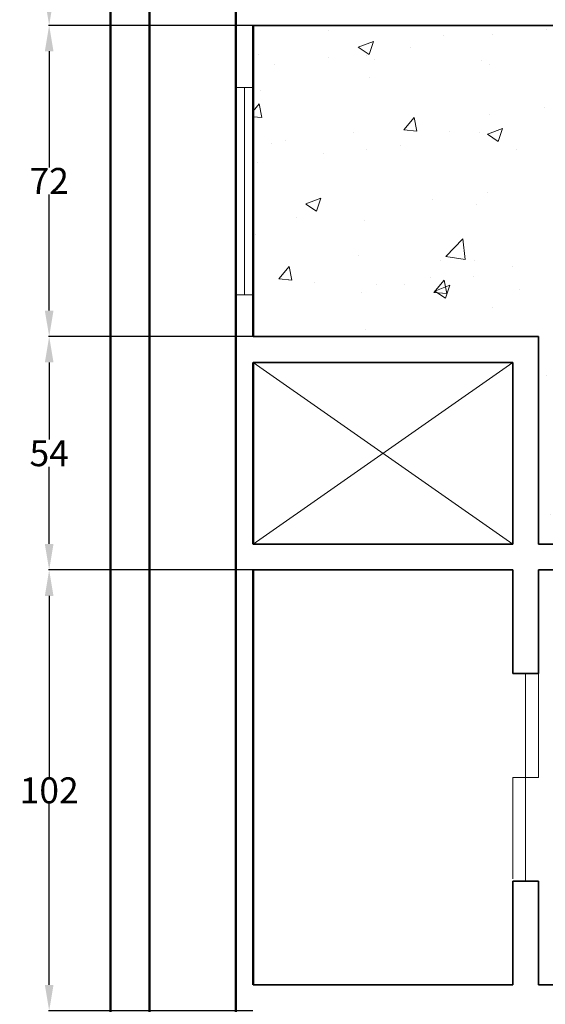
# Model space of a CAD drawing. Units: inches. Extents: x 910 to 1553, y 598 to 1516.
# Tile 3 of 6: x 910 to 1031, y 1079 to 1307. Entities that reach past the tile are written whole.
import ezdxf

# ---------------------------------------------------------------- set-up
doc = ezdxf.new("R2010")
doc.units = ezdxf.units.IN
doc.header["$MEASUREMENT"] = 0
for name, color, linetype, lineweight in [('A-ANNO-DIMS', 2, 'Continuous', 18), ('A-FLOR-OPEN', 8, 'Continuous', 13), ('A-FLOR-PATT', 252, 'Continuous', 13), ('doors', 2, 'Continuous', 18), ('Inner wall', 230, 'Continuous', 35), ('outer wall', 231, 'Continuous', 50), ('windows', 6, 'Continuous', 18)]:
    doc.layers.add(name, color=color, linetype=linetype, lineweight=lineweight)
doc.styles.get("Standard").update_dxf_attribs({"font": 'arial.ttf'})
doc.dimstyles.get("Standard").update_dxf_attribs({"dimtxt": 6, "dimasz": 6, "dimexe": 0.18, "dimexo": 0.0625, "dimgap": 0.09, "dimtad": 0, "dimtih": 1, "dimtoh": 1, "dimdec": 0, "dimzin": 0, "dimdsep": 46, "dimlunit": 3, "dimtxsty": 'Standard', "dimcen": 0.09, "dimadec": 0, "dimazin": 0, "dimtfac": 1, "dimtdec": 0, "dimtofl": 0, "dimtmove": 0, "dimatfit": 3, "dimfxl": 1, "dimtolj": 1, "dimtzin": 0, "dimarcsym": 0})

# ---------------------------------------------------------------- blocks, each defined once
blk = doc.blocks.new('*D66')
at = {"layer": 'A-ANNO-DIMS', "color": 0, "lineweight": -2, "transparency": 16777216}
for p, q in [((963.64, 1179.97), (916.34, 1179.97)), ((916.52, 1173.97), (916.52, 1132.12)), ((916.52, 1083.97), (916.52, 1125.82)), ((963.64, 1077.97), (916.34, 1077.97))]:
    blk.add_line(p, q, dxfattribs=at)
for points in [[(915.52, 1173.97), (917.52, 1173.97), (916.52, 1179.97)], [(915.52, 1083.97), (917.52, 1083.97), (916.52, 1077.97)]]:
    blk.add_solid(points, dxfattribs=at)
at = {"layer": 'Defpoints', "color": 0, "lineweight": -2, "transparency": 16777216}
for p in [(916.52, 1179.97), (963.7, 1179.97), (963.7, 1077.97)]:
    blk.add_point(p, dxfattribs=at)
at = {"layer": 'A-ANNO-DIMS', "color": 0, "transparency": 16777216, "insert": (916.52, 1128.97), "char_height": 6, "attachment_point": 5}
blk.add_mtext('\\A1;102', dxfattribs=at)
blk = doc.blocks.new('*D67')
at = {"layer": 'A-ANNO-DIMS', "color": 0, "lineweight": -2, "transparency": 16777216}
for p, q in [((963.64, 1233.97), (916.34, 1233.97)), ((916.52, 1227.97), (916.52, 1210.11)), ((916.52, 1185.97), (916.52, 1203.83)), ((963.64, 1179.97), (916.34, 1179.97))]:
    blk.add_line(p, q, dxfattribs=at)
for points in [[(915.52, 1227.97), (917.52, 1227.97), (916.52, 1233.97)], [(915.52, 1185.97), (917.52, 1185.97), (916.52, 1179.97)]]:
    blk.add_solid(points, dxfattribs=at)
at = {"layer": 'Defpoints', "color": 0, "lineweight": -2, "transparency": 16777216}
for p in [(916.52, 1233.97), (963.7, 1233.97), (963.7, 1179.97)]:
    blk.add_point(p, dxfattribs=at)
at = {"layer": 'A-ANNO-DIMS', "color": 0, "transparency": 16777216, "insert": (916.52, 1206.97), "char_height": 6, "attachment_point": 5}
blk.add_mtext('\\A1;54', dxfattribs=at)
blk = doc.blocks.new('*D68')
at = {"layer": 'A-ANNO-DIMS', "color": 0, "lineweight": -2, "transparency": 16777216}
for p, q in [((963.64, 1305.97), (916.34, 1305.97)), ((916.52, 1299.97), (916.52, 1273.07)), ((916.52, 1239.97), (916.52, 1266.87)), ((963.64, 1233.97), (916.34, 1233.97))]:
    blk.add_line(p, q, dxfattribs=at)
for points in [[(915.52, 1299.97), (917.52, 1299.97), (916.52, 1305.97)], [(915.52, 1239.97), (917.52, 1239.97), (916.52, 1233.97)]]:
    blk.add_solid(points, dxfattribs=at)
at = {"layer": 'Defpoints', "color": 0, "lineweight": -2, "transparency": 16777216}
for p in [(916.52, 1305.97), (963.7, 1305.97), (963.7, 1233.97)]:
    blk.add_point(p, dxfattribs=at)
at = {"layer": 'A-ANNO-DIMS', "color": 0, "transparency": 16777216, "insert": (916.52, 1269.97), "char_height": 6, "attachment_point": 5}
blk.add_mtext('\\A1;72', dxfattribs=at)
blk = doc.blocks.new('*D69')
at = {"layer": 'A-ANNO-DIMS', "color": 0, "lineweight": -2, "transparency": 16777216}
for p, q in [((963.64, 1353.97), (916.34, 1353.97)), ((916.52, 1347.97), (916.52, 1333.12)), ((916.52, 1311.97), (916.52, 1326.82)), ((963.64, 1305.97), (916.34, 1305.97))]:
    blk.add_line(p, q, dxfattribs=at)
for points in [[(915.52, 1347.97), (917.52, 1347.97), (916.52, 1353.97)], [(915.52, 1311.97), (917.52, 1311.97), (916.52, 1305.97)]]:
    blk.add_solid(points, dxfattribs=at)
at = {"layer": 'Defpoints', "color": 0, "lineweight": -2, "transparency": 16777216}
for p in [(916.52, 1353.97), (963.7, 1353.97), (963.7, 1305.97)]:
    blk.add_point(p, dxfattribs=at)
at = {"layer": 'A-ANNO-DIMS', "color": 0, "transparency": 16777216, "insert": (916.52, 1329.97), "char_height": 6, "attachment_point": 5}
blk.add_mtext('\\A1;48', dxfattribs=at)

msp = doc.modelspace()

# ---------------------------------------------------------------- hatches: boundary and pattern name
at = {"layer": 'A-FLOR-PATT'}
h = msp.add_hatch(dxfattribs=at)
h.set_pattern_fill('AR-CONC', color=256, scale=5)
h.paths.add_polyline_path([(1149.7, 1305.969), (1029.7, 1305.969), (1023.7, 1305.969), (963.7, 1305.969), (963.7, 1233.969), (1023.7, 1233.969), (1029.7, 1233.969), (1029.7, 1185.969), (1149.7, 1185.969), (1149.7, 1188.289), (1151.2, 1188.289), (1136.2, 1214.269), (1137.337, 1214.926), (1137.352, 1214.901, -0.107869), (1149.7, 1218.251)])
h.paths.add_polyline_path([(1037.415, 1285.215), (1068.009, 1285.215), (1068.009, 1259.257), (1067.082, 1259.257), (1067.082, 1258.33), (1066.155, 1258.33), (1066.155, 1259.257), (1037.415, 1259.257)], flags=16)
h.paths.add_polyline_path([(1033.378, 1259.726), (1032.395, 1260.709), (1033.378, 1261.693), (1032.395, 1262.676), (1033.378, 1263.659), (1032.395, 1264.642), (1033.378, 1265.626), (1032.395, 1266.609), (1033.378, 1267.592), (1032.395, 1268.576), (1033.378, 1269.559), (1032.395, 1270.542), (1033.378, 1271.526), (1032.395, 1272.509), (1033.378, 1273.492), (1032.395, 1274.476), (1033.378, 1275.459), (1032.395, 1276.442), (1033.378, 1277.426), (1032.395, 1278.409), (1033.378, 1279.392), (1032.395, 1280.376), (1033.378, 1281.359), (1032.395, 1282.342), (1033.378, 1283.326), (1032.395, 1284.309), (1033.378, 1285.292), (1032.395, 1286.275), (1033.378, 1287.259), (1032.395, 1288.242), (1034.362, 1290.209), (1035.345, 1289.225), (1036.328, 1290.209), (1037.312, 1289.225), (1038.295, 1290.209), (1039.278, 1289.225), (1040.262, 1290.209), (1041.245, 1289.225), (1042.228, 1290.209), (1043.212, 1289.225), (1044.195, 1290.209), (1045.178, 1289.225), (1046.162, 1290.209), (1047.145, 1289.225), (1048.128, 1290.209), (1049.111, 1289.225), (1050.095, 1290.209), (1051.078, 1289.225), (1052.061, 1290.209), (1053.045, 1289.225), (1054.028, 1290.209), (1055.011, 1289.225), (1055.995, 1290.209), (1056.978, 1289.225), (1057.961, 1290.209), (1058.945, 1289.225), (1059.928, 1290.209), (1060.911, 1289.225), (1061.895, 1290.209), (1062.878, 1289.225), (1063.861, 1290.209), (1064.845, 1289.225), (1065.828, 1290.209), (1066.811, 1289.225), (1067.795, 1290.209), (1068.778, 1289.225), (1069.761, 1290.209), (1070.745, 1289.225), (1071.728, 1290.209), (1072.711, 1289.225), (1073.694, 1290.209), (1074.678, 1289.225), (1075.661, 1290.209), (1076.644, 1289.225), (1077.628, 1290.209), (1078.611, 1289.225), (1079.594, 1290.209), (1080.578, 1289.225), (1081.561, 1290.209), (1082.544, 1289.225), (1083.528, 1290.209), (1084.511, 1289.225), (1085.494, 1290.209), (1086.478, 1289.225), (1087.461, 1290.209), (1088.444, 1289.225), (1089.428, 1290.209), (1090.411, 1289.225), (1091.394, 1290.209), (1092.378, 1289.225), (1093.361, 1290.209), (1094.344, 1289.225), (1095.327, 1290.209), (1096.311, 1289.225), (1097.294, 1290.209), (1098.277, 1289.225), (1099.261, 1290.209), (1100.244, 1289.225), (1101.227, 1290.209), (1102.211, 1289.225), (1103.194, 1290.209), (1104.177, 1289.225), (1105.161, 1290.209), (1106.144, 1289.225), (1107.127, 1290.209), (1108.111, 1289.225), (1109.094, 1290.209), (1110.077, 1289.225), (1111.061, 1290.209), (1112.044, 1289.225), (1113.027, 1290.209), (1114.011, 1289.225), (1114.994, 1290.209), (1115.977, 1289.225), (1116.961, 1290.209), (1117.944, 1289.225), (1118.927, 1290.209), (1119.91, 1289.225), (1120.894, 1290.209), (1121.877, 1289.225), (1122.86, 1290.209), (1123.844, 1289.225), (1124.827, 1290.209), (1125.81, 1289.225), (1126.794, 1290.209), (1127.777, 1289.225), (1128.76, 1290.209), (1130.727, 1288.242), (1129.744, 1287.259), (1130.727, 1286.275), (1129.744, 1285.292), (1130.727, 1284.309), (1129.744, 1283.326), (1130.727, 1282.342), (1129.744, 1281.359), (1130.727, 1280.376), (1129.744, 1279.392), (1130.727, 1278.409), (1129.744, 1277.426), (1130.727, 1276.442), (1129.744, 1275.459), (1130.727, 1274.476), (1129.744, 1273.492), (1130.727, 1272.509), (1129.744, 1271.526), (1130.727, 1270.542), (1129.744, 1269.559), (1130.727, 1268.576), (1129.744, 1267.592), (1130.727, 1266.609), (1129.744, 1265.626), (1130.727, 1264.642), (1128.76, 1262.676), (1127.777, 1263.659), (1128.76, 1264.642), (1127.777, 1265.626), (1128.76, 1266.609), (1127.777, 1267.592), (1128.76, 1268.576), (1127.777, 1269.559), (1128.76, 1270.542), (1127.777, 1271.526), (1128.76, 1272.509), (1127.777, 1273.492), (1128.76, 1274.476), (1127.777, 1275.459), (1128.76, 1276.442), (1127.777, 1277.426), (1128.76, 1278.409), (1127.777, 1279.392), (1128.76, 1280.376), (1127.777, 1281.359), (1128.76, 1282.342), (1127.777, 1283.326), (1128.76, 1284.309), (1127.342, 1285.727), (1125.81, 1287.259), (1124.827, 1286.275), (1123.844, 1287.259), (1122.86, 1286.275), (1121.877, 1287.259), (1120.894, 1286.275), (1119.91, 1287.259), (1118.927, 1286.275), (1117.944, 1287.259), (1116.961, 1286.275), (1115.977, 1287.259), (1114.994, 1286.275), (1114.011, 1287.259), (1113.027, 1286.275), (1112.044, 1287.259), (1111.061, 1286.275), (1110.077, 1287.259), (1109.094, 1286.275), (1108.111, 1287.259), (1107.127, 1286.275), (1106.144, 1287.259), (1105.161, 1286.275), (1104.177, 1287.259), (1103.194, 1286.275), (1102.211, 1287.259), (1101.227, 1286.275), (1100.244, 1287.259), (1099.261, 1286.275), (1098.277, 1287.259), (1097.294, 1286.275), (1096.311, 1287.259), (1095.327, 1286.275), (1094.344, 1287.259), (1093.361, 1286.275), (1092.378, 1287.259), (1091.394, 1286.275), (1090.411, 1287.259), (1089.428, 1286.275), (1088.444, 1287.259), (1087.461, 1286.275), (1086.478, 1287.259), (1085.494, 1286.275), (1084.511, 1287.259), (1083.528, 1286.275), (1082.544, 1287.259), (1081.561, 1286.275), (1080.578, 1287.259), (1079.594, 1286.275), (1078.611, 1287.259), (1077.628, 1286.275), (1076.644, 1287.259), (1075.661, 1286.275), (1074.678, 1287.259), (1073.694, 1286.275), (1072.711, 1287.259), (1071.728, 1286.275), (1070.745, 1287.259), (1069.761, 1286.275), (1068.778, 1287.259), (1067.795, 1286.275), (1066.811, 1287.259), (1065.828, 1286.275), (1064.845, 1287.259), (1063.861, 1286.275), (1062.878, 1287.259), (1061.895, 1286.275), (1060.911, 1287.259), (1059.928, 1286.275), (1058.945, 1287.259), (1057.961, 1286.275), (1056.978, 1287.259), (1055.995, 1286.275), (1055.011, 1287.259), (1054.028, 1286.275), (1053.045, 1287.259), (1052.061, 1286.275), (1051.078, 1287.259), (1050.095, 1286.275), (1049.111, 1287.259), (1048.128, 1286.275), (1047.145, 1287.259), (1046.162, 1286.275), (1045.178, 1287.259), (1044.195, 1286.275), (1043.212, 1287.259), (1042.228, 1286.275), (1041.245, 1287.259), (1040.262, 1286.275), (1039.278, 1287.259), (1038.295, 1286.275), (1037.312, 1287.259), (1035.345, 1285.292), (1036.328, 1284.309), (1035.345, 1283.326), (1036.328, 1282.342), (1035.345, 1281.359), (1036.328, 1280.376), (1035.345, 1279.392), (1036.328, 1278.409), (1035.345, 1277.426), (1036.328, 1276.442), (1035.345, 1275.459), (1036.328, 1274.476), (1035.345, 1273.492), (1036.328, 1272.509), (1035.345, 1271.526), (1036.328, 1270.542), (1035.345, 1269.559), (1036.328, 1268.576), (1035.345, 1267.592), (1036.328, 1266.609), (1035.345, 1265.626), (1036.328, 1264.642), (1035.345, 1263.659), (1036.328, 1262.676), (1035.345, 1261.693), (1036.328, 1260.709), (1035.345, 1259.726), (1034.362, 1260.709)], flags=16)
h.paths.add_polyline_path([(1107.873, 1261.111), (1107.873, 1262.038), (1111.582, 1262.038), (1111.582, 1262.965), (1106.019, 1262.965), (1068.936, 1262.965), (1068.936, 1285.215), (1126.415, 1285.215), (1126.415, 1262.965), (1125.488, 1262.965), (1125.488, 1262.965), (1119.925, 1262.965), (1119.925, 1262.038), (1123.634, 1262.038), (1123.634, 1261.111)], flags=16)
h.paths.add_polyline_path([(1038.223, 1252.226), (1042.156, 1256.159), (1046.09, 1252.226), (1050.023, 1256.159), (1053.956, 1252.226), (1057.889, 1256.159), (1061.823, 1252.226), (1067.927, 1258.33), (1069.689, 1260.092), (1073.622, 1256.159), (1077.556, 1260.092), (1081.489, 1256.159), (1085.422, 1260.092), (1089.356, 1256.159), (1093.289, 1260.092), (1097.222, 1256.159), (1101.155, 1260.092), (1105.089, 1256.159), (1109.022, 1260.092), (1112.955, 1256.159), (1116.889, 1260.092), (1124.755, 1252.226), (1120.822, 1248.292), (1124.755, 1244.359), (1120.822, 1240.426), (1124.755, 1236.493), (1120.822, 1232.559), (1123.791, 1229.59), (1126.415, 1229.59), (1126.415, 1207.34), (1037.415, 1207.34), (1037.415, 1229.59), (1039.187, 1229.59), (1042.156, 1232.559), (1038.223, 1236.493), (1042.156, 1240.426), (1038.223, 1244.359), (1042.156, 1248.292)], flags=16)
h.paths.add_polyline_path([(1036.328, 1227.276), (1035.345, 1226.293), (1036.328, 1225.31), (1035.345, 1224.326), (1036.328, 1223.343), (1035.345, 1222.36), (1036.328, 1221.376), (1035.345, 1220.393), (1036.328, 1219.41), (1035.345, 1218.426), (1036.328, 1217.443), (1035.345, 1216.46), (1036.328, 1215.476), (1035.345, 1214.493), (1036.328, 1213.51), (1035.345, 1212.527), (1036.328, 1211.543), (1035.345, 1210.56), (1036.328, 1209.577), (1035.345, 1208.593), (1036.328, 1207.61), (1035.345, 1206.627), (1036.328, 1205.643), (1037.312, 1206.627), (1038.295, 1205.643), (1039.278, 1206.627), (1040.262, 1205.643), (1041.245, 1206.627), (1042.228, 1205.643), (1043.212, 1206.627), (1044.195, 1205.643), (1045.178, 1206.627), (1046.162, 1205.643), (1047.145, 1206.627), (1048.128, 1205.643), (1049.111, 1206.627), (1050.095, 1205.643), (1051.078, 1206.627), (1052.061, 1205.643), (1053.045, 1206.627), (1054.028, 1205.643), (1055.011, 1206.627), (1055.995, 1205.643), (1056.978, 1206.627), (1057.961, 1205.643), (1058.945, 1206.627), (1059.928, 1205.643), (1060.911, 1206.627), (1061.895, 1205.643), (1062.878, 1206.627), (1064.845, 1204.66), (1062.878, 1202.693), (1061.895, 1203.677), (1060.911, 1202.693), (1059.928, 1203.677), (1058.945, 1202.693), (1057.961, 1203.677), (1056.978, 1202.693), (1055.995, 1203.677), (1055.011, 1202.693), (1054.028, 1203.677), (1053.045, 1202.693), (1052.061, 1203.677), (1051.078, 1202.693), (1050.095, 1203.677), (1049.111, 1202.693), (1048.128, 1203.677), (1047.145, 1202.693), (1046.162, 1203.677), (1045.178, 1202.693), (1044.195, 1203.677), (1043.212, 1202.693), (1042.228, 1203.677), (1041.245, 1202.693), (1040.262, 1203.677), (1039.278, 1202.693), (1038.295, 1203.677), (1037.312, 1202.693), (1036.328, 1203.677), (1035.345, 1202.693), (1034.362, 1203.677), (1033.378, 1202.693), (1032.395, 1203.677), (1033.378, 1204.66), (1032.395, 1205.643), (1033.378, 1206.627), (1032.395, 1207.61), (1033.378, 1208.593), (1032.395, 1209.577), (1033.378, 1210.56), (1032.395, 1211.543), (1033.378, 1212.527), (1032.395, 1213.51), (1033.378, 1214.493), (1032.395, 1215.476), (1033.378, 1216.46), (1032.395, 1217.443), (1033.378, 1218.426), (1032.395, 1219.41), (1033.378, 1220.393), (1032.395, 1221.376), (1033.378, 1222.36), (1032.395, 1223.343), (1033.378, 1224.326), (1032.395, 1225.31), (1033.378, 1226.293), (1032.395, 1227.276), (1034.362, 1229.243)], flags=16)
h.paths.add_polyline_path([(1068.472, 1226.809), (1095.358, 1226.809, -0.4142136), (1096.748, 1225.419), (1096.748, 1208.731, -0.4142136), (1095.358, 1207.34), (1068.472, 1207.34, -0.4142136), (1067.082, 1208.731), (1067.082, 1225.419, -0.4142136)], flags=16)
h.paths.add_polyline_path([(1068.472, 1224.491, -0.4142136), (1069.399, 1225.419), (1080.293, 1225.419, -0.4142136), (1081.22, 1224.491), (1081.22, 1213.366, -0.4142136), (1080.293, 1212.439), (1069.399, 1212.439, -0.4142136), (1068.472, 1213.366)], flags=0)
h.paths.add_polyline_path([(1074.498, 1218.929, -1), (1075.425, 1218.929, -1)], flags=0)
h.paths.add_polyline_path([(1082.61, 1224.491, -0.4142136), (1083.537, 1225.419), (1094.431, 1225.419, -0.4142136), (1095.358, 1224.491), (1095.358, 1213.366, -0.4142136), (1094.431, 1212.439), (1083.537, 1212.439, -0.4142136), (1082.61, 1213.366)], flags=0)
h.paths.add_polyline_path([(1088.405, 1218.929, -1), (1089.332, 1218.929, -1)], flags=0)
h.paths.add_polyline_path([(1114.363, 1268.528, -1), (1108.8, 1268.528, -1)], flags=0)
h.paths.add_polyline_path([(1107.873, 1276.872, -1), (1115.29, 1276.872, -1)], flags=0)
h.paths.add_polyline_path([(1113.436, 1268.528, -1), (1109.727, 1268.528, -1)], flags=0)
h.paths.add_polyline_path([(1114.363, 1276.872, -1), (1108.8, 1276.872, -1)], flags=0)
h.paths.add_polyline_path([(1112.509, 1268.528, -1), (1110.655, 1268.528, -1)], flags=0)
h.paths.add_polyline_path([(1113.436, 1276.872, -1), (1109.727, 1276.872, -1)], flags=0)
h.paths.add_polyline_path([(1112.509, 1276.872, -1), (1110.655, 1276.872, -1)], flags=0)
h.paths.add_polyline_path([(1100.244, 1206.627), (1101.227, 1205.643), (1102.211, 1206.627), (1103.194, 1205.643), (1104.177, 1206.627), (1105.161, 1205.643), (1106.144, 1206.627), (1107.127, 1205.643), (1108.111, 1206.627), (1109.094, 1205.643), (1110.077, 1206.627), (1111.061, 1205.643), (1112.044, 1206.627), (1113.027, 1205.643), (1114.011, 1206.627), (1114.994, 1205.643), (1115.977, 1206.627), (1116.961, 1205.643), (1117.944, 1206.627), (1118.927, 1205.643), (1119.91, 1206.627), (1120.894, 1205.643), (1121.877, 1206.627), (1122.86, 1205.643), (1123.844, 1206.627), (1124.827, 1205.643), (1125.81, 1206.627), (1126.794, 1205.643), (1128.76, 1207.61), (1127.777, 1208.593), (1128.76, 1209.577), (1127.777, 1210.56), (1128.76, 1211.543), (1127.777, 1212.527), (1128.76, 1213.51), (1127.777, 1214.493), (1128.76, 1215.476), (1127.777, 1216.46), (1128.76, 1217.443), (1127.777, 1218.426), (1128.76, 1219.41), (1127.777, 1220.393), (1128.76, 1221.376), (1127.777, 1222.36), (1128.76, 1223.343), (1127.777, 1224.326), (1128.76, 1225.31), (1127.777, 1226.293), (1128.76, 1227.276), (1127.777, 1228.26), (1128.76, 1229.243), (1130.727, 1227.276), (1129.744, 1226.293), (1130.727, 1225.31), (1129.744, 1224.326), (1130.727, 1223.343), (1129.744, 1222.36), (1130.727, 1221.376), (1129.744, 1220.393), (1130.727, 1219.41), (1129.744, 1218.426), (1130.727, 1217.443), (1129.744, 1216.46), (1130.727, 1215.476), (1129.744, 1214.493), (1130.727, 1213.51), (1129.744, 1212.527), (1130.727, 1211.543), (1129.744, 1210.56), (1130.727, 1209.577), (1129.744, 1208.593), (1130.727, 1207.61), (1129.744, 1206.627), (1130.727, 1205.643), (1129.744, 1204.66), (1130.727, 1203.677), (1129.744, 1202.693), (1128.76, 1203.677), (1127.777, 1202.693), (1126.794, 1203.677), (1125.81, 1202.693), (1124.827, 1203.677), (1123.844, 1202.693), (1122.86, 1203.677), (1121.877, 1202.693), (1120.894, 1203.677), (1119.91, 1202.693), (1118.927, 1203.677), (1117.944, 1202.693), (1116.961, 1203.677), (1115.977, 1202.693), (1114.994, 1203.677), (1114.011, 1202.693), (1113.027, 1203.677), (1112.044, 1202.693), (1111.061, 1203.677), (1110.077, 1202.693), (1109.094, 1203.677), (1108.111, 1202.693), (1107.127, 1203.677), (1106.144, 1202.693), (1105.161, 1203.677), (1104.177, 1202.693), (1103.194, 1203.677), (1102.211, 1202.693), (1101.227, 1203.677), (1100.244, 1202.693), (1098.277, 1204.66)], flags=16)
h.paths.add_polyline_path([(1123.634, 1268.528, -1), (1116.217, 1268.528, -1)], flags=0)
h.paths.add_polyline_path([(1122.707, 1268.528, -1), (1117.144, 1268.528, -1)], flags=0)
h.paths.add_polyline_path([(1121.779, 1268.528, -1), (1118.071, 1268.528, -1)], flags=0)
h.paths.add_polyline_path([(1122.707, 1276.872, -1), (1117.144, 1276.872, -1)], flags=0)
h.paths.add_polyline_path([(1120.852, 1268.528, -1), (1118.998, 1268.528, -1)], flags=0)
h.paths.add_polyline_path([(1121.779, 1276.872, -1), (1118.071, 1276.872, -1)], flags=0)
h.paths.add_polyline_path([(1120.852, 1276.872, -1), (1118.998, 1276.872, -1)], flags=0)

# ---------------------------------------------------------------- linework, layer by layer
at = {"layer": 'A-FLOR-OPEN'}
for p, q in [((1023.7, 1227.969), (963.7, 1185.969)), ((963.7, 1227.969), (1023.7, 1185.969))]:
    msp.add_line(p, q, dxfattribs=at)
at = {"layer": 'doors'}
for p, q in [((1026.7, 1155.969), (1026.7, 1107.969)), ((1029.7, 1155.969), (1029.7, 1131.969)), ((1023.7, 1131.969), (1023.7, 1108.5)), ((1029.7, 1131.969), (1023.7, 1131.969))]:
    msp.add_line(p, q, dxfattribs=at)
at = {"layer": 'Inner wall'}
for p, q in [((1023.7, 1305.969), (963.7, 1305.969)), ((1023.7, 1305.969), (1029.7, 1305.969)), ((1149.7, 1305.969), (1029.7, 1305.969)), ((1023.7, 1233.969), (963.7, 1233.969)), ((1023.7, 1233.969), (1029.7, 1233.969)), ((1029.7, 1233.969), (1029.7, 1185.969)), ((1023.7, 1227.969), (963.7, 1227.969)), ((1023.7, 1227.969), (1023.7, 1185.969)), ((1023.7, 1185.969), (963.7, 1185.969)), ((1149.7, 1185.969), (1029.7, 1185.969)), ((1023.7, 1179.969), (963.7, 1179.969)), ((1023.7, 1179.969), (1023.7, 1155.969)), ((1029.7, 1179.969), (1029.7, 1155.969)), ((1149.7, 1179.969), (1029.7, 1179.969)), ((1029.7, 1155.969), (1023.7, 1155.969)), ((1029.7, 1107.969), (1023.7, 1107.969)), ((1023.7, 1107.969), (1023.7, 1083.969)), ((1029.7, 1107.969), (1029.7, 1083.969)), ((1023.7, 1083.969), (963.7, 1083.969)), ((1149.7, 1083.969), (1029.7, 1083.969))]:
    msp.add_line(p, q, dxfattribs=at)
at = {"layer": 'outer wall'}
for p, q in [((939.7, 1479.969), (939.7, 633.969)), ((959.7, 1449.969), (959.7, 681.969)), ((963.7, 1305.969), (963.7, 1233.969)), ((963.7, 1227.969), (963.7, 1185.969)), ((963.7, 1179.969), (963.7, 1083.969))]:
    msp.add_line(p, q, dxfattribs=at)
msp.add_lwpolyline([(1530.7, 1488.969), (930.7, 1488.969), (930.7, 624.969), (1530.7, 624.969)], close=True, dxfattribs=at)
at = {"layer": 'windows'}
for p, q in [((959.7, 1291.602), (963.7, 1291.602)), ((959.7, 1243.602), (959.7, 1291.602)), ((961.7, 1291.602), (961.7, 1243.602)), ((963.7, 1291.602), (963.7, 1243.602)), ((963.7, 1243.602), (959.7, 1243.602))]:
    msp.add_line(p, q, dxfattribs=at)

# ---------------------------------------------------------------- dimensions: what is measured, and where the dimension line sits
at = {"layer": 'A-ANNO-DIMS'}
for base, p1, p2, picture, middle in [((916.52, 1353.969), (963.7, 1305.969), (963.7, 1353.969), '*D69', (916.52, 1329.969)), ((916.52, 1305.969), (963.7, 1233.969), (963.7, 1305.969), '*D68', (916.52, 1269.969)), ((916.52, 1233.969), (963.7, 1179.969), (963.7, 1233.969), '*D67', (916.52, 1206.969)), ((916.52, 1179.969), (963.7, 1077.969), (963.7, 1179.969), '*D66', (916.52, 1128.969))]:
    dim = msp.add_linear_dim(base=base, p1=p1, p2=p2, angle=90, dimstyle='Standard', override={"dimdec": 0, "dimlfac": 1, "dimrnd": 0, "dimzin": 0, "dimdsep": 46, "dimlunit": 2}, dxfattribs=at)
    dim.commit()
    dim.dimension.update_dxf_attribs({"geometry": picture, "text_midpoint": middle})

doc.saveas('drawing.dxf')
